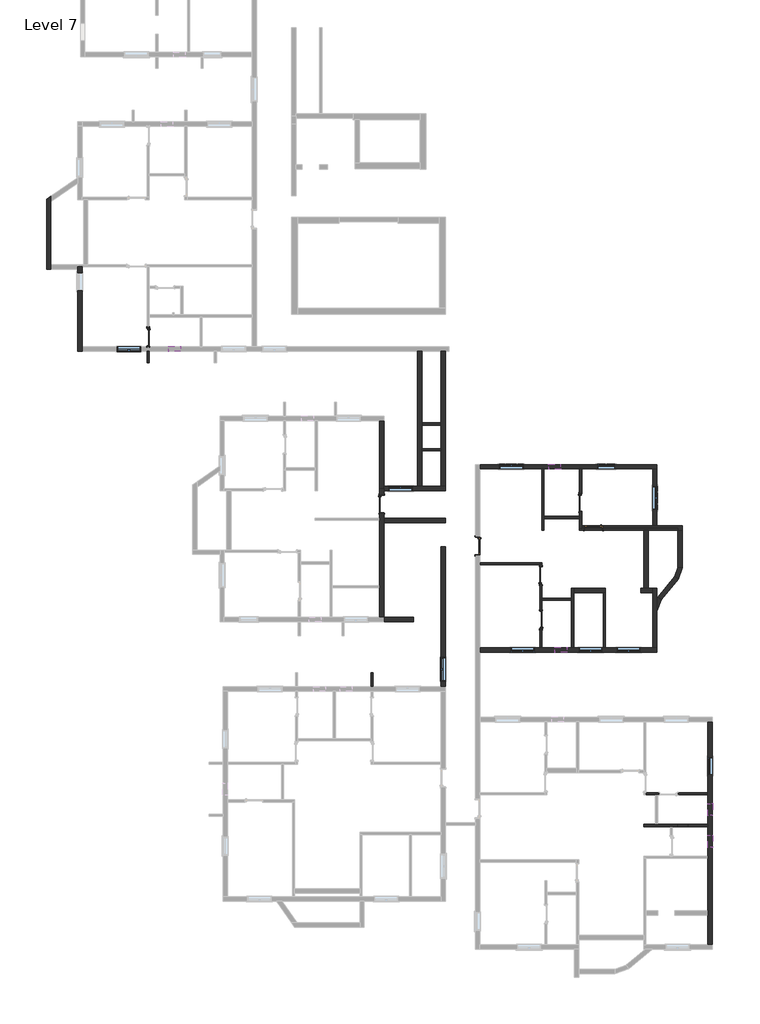
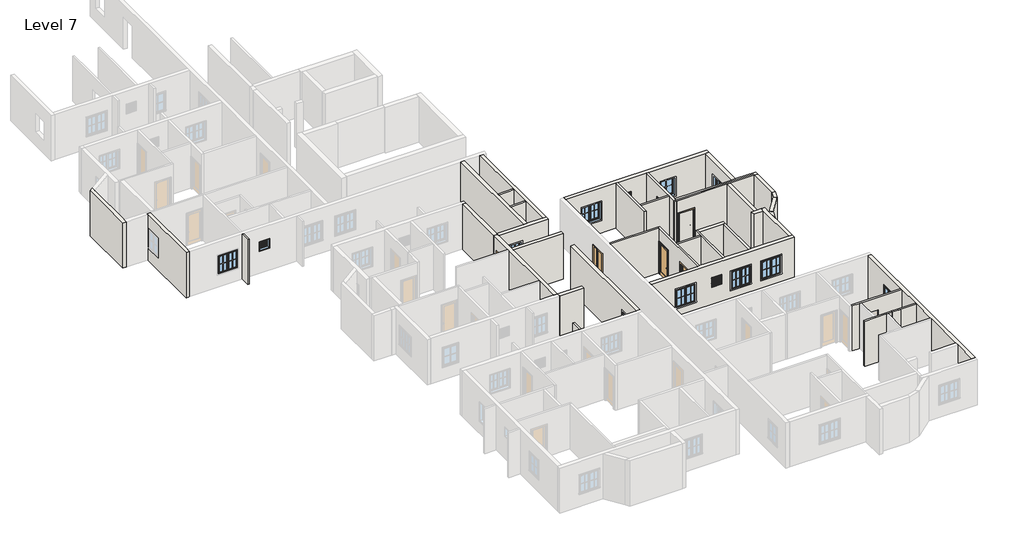
# One storey, part 3 of 7: 39 walls, 15 windows, 7 doors.
"""IFC4 building model written with IfcOpenShell, lengths in millimetres."""

from ifc_helpers import new_model, si_unit, point, frame, frame_2d, origin, place, context, project, spatial, polyline, circle_curve, trimmed, segment, composite_curve, outline, extrude, faceted_brep, transform, mapped, element, save
from components import door_3c6ab76a, door_a3feeac7, door_3b97b8e7, door_868ee8a9, window_272f20d6, window_casement_double_4_x_4_af3140d2, window_f2d8fef0

model = new_model("IFC4")

# Units and contexts
model_context = context("Model", 3, world=origin())
ifc_project = project(units=[si_unit("LENGTHUNIT", "METRE", prefix="MILLI")], contexts=[model_context])

# Site, building, storey
site = spatial("IfcSite", under=ifc_project)
building = spatial("IfcBuilding", under=site)
storey = spatial("IfcBuildingStorey", under=building, Name="Level 7", Elevation=9601.2)

# Doors
placement = place(None, origin())
door_shape = door_3c6ab76a(model_context)
element("IfcDoor", 1, ObjectType="Door-Interior-Single-1_Panel-Wood : 2'6\" x 7' door", at=placement, inside=storey, context=model_context, shape_type="MappedRepresentation", body=[
    mapped(door_shape, transform((-11252.4759469, 2064.0461172, 9601.2), x_axis=(0.0, -1.0, 0.0), y_axis=(1.0, 0.0, 0.0), z_axis=(0.0, 0.0, 1.0))),
])
door_2_shape = door_a3feeac7(model_context)
element("IfcDoor", 2, ObjectType="Door-Interior-Single-1_Panel-Wood : 2'6\" x 7' door", at=placement, inside=storey, context=model_context, shape_type="MappedRepresentation", body=[
    mapped(door_2_shape, transform((11042.3740531, -6465.2997229, 9601.2), x_axis=(0.0, -1.0, 0.0), y_axis=(1.0, 0.0, 0.0), z_axis=(0.0, 0.0, 1.0))),
])
element("IfcDoor", 3, ObjectType="Door-Interior-Single-1_Panel-Wood : 2'6\" x 7' door", at=placement, inside=storey, context=model_context, shape_type="MappedRepresentation", body=[
    mapped(door_2_shape, transform((9004.0240531, -12510.4997229, 9601.2), x_axis=(0.0, 1.0, 0.0), y_axis=(-1.0, 0.0, 0.0), z_axis=(0.0, 0.0, 1.0))),
])
element("IfcDoor", 4, ObjectType="Door-Interior-Single-1_Panel-Wood : 36\" x 84\"", at=placement, inside=storey, context=model_context, shape_type="MappedRepresentation", body=[
    mapped(door_shape, transform((8997.6740531, -10224.4997229, 9601.2), x_axis=(0.0, 1.0, 0.0), y_axis=(-1.0, 0.0, 0.0), z_axis=(0.0, 0.0, 1.0))),
])
door_3_shape = door_3b97b8e7(model_context)
element("IfcDoor", 5, ObjectType="Door-Interior-Single-1_Panel-Wood : 36\" x 84\"", at=placement, inside=storey, context=model_context, shape_type="MappedRepresentation", body=[
    mapped(door_3_shape, transform((5733.7740531, -8700.4997229, 9601.2), x_axis=(0.0, -1.0, 0.0), y_axis=(1.0, 0.0, 0.0), z_axis=(0.0, 0.0, 1.0))),
])
door_4_shape = door_868ee8a9(model_context)
element("IfcDoor", 6, ObjectType="Door-Interior-Single-1_Panel-Wood : 36\" x 84\"", at=placement, inside=storey, context=model_context, shape_type="MappedRepresentation", body=[
    mapped(door_4_shape, transform((787.1240531, -6537.0288828, 9601.2), x_axis=(0.0, -1.0, 0.0), y_axis=(1.0, 0.0, 0.0), z_axis=(0.0, 0.0, 1.0))),
])
element("IfcDoor", 7, ObjectType="Door-Interior-Single-1_Panel-Wood : 36\" x 84\"", at=placement, inside=storey, context=model_context, shape_type="MappedRepresentation", body=[
    mapped(door_4_shape, transform((11712.2990531, -7776.5747229, 9601.2), x_axis=(-1.0, 0.0, 0.0), y_axis=(0.0, -1.0, 0.0), z_axis=(0.0, 0.0, 1.0))),
])

# Walls
element("IfcWall", 8, ObjectType="4.5\" wall", at=placement, inside=storey, context=model_context, shape_type="SweptSolid", body=[
    extrude(outline(polyline([(-11312.8009469, 730.5461172), (-11312.8009469, 1340.1461172), (-11198.5009469, 1340.1461172), (-11198.5009469, 730.5461172), (-11312.8009469, 730.5461172)])), frame((0.0, 0.0, 9601.2), z_axis=(0.0, 0.0, 1.0), x_axis=(1.0, 0.0, 0.0)), (0.0, 0.0, 1.0), 3048.0),
])
element("IfcWall", 9, ObjectType="4.5\" wall", at=placement, inside=storey, context=model_context, shape_type="SweptSolid", body=[
    extrude(outline(polyline([(3850.9990531, -3803.3538828), (2860.3990531, -3803.3538828), (2860.3990531, -3689.0538828), (3850.9990531, -3689.0538828), (3850.9990531, -3803.3538828)])), frame((0.0, 0.0, 9601.2), z_axis=(0.0, 0.0, 1.0), x_axis=(1.0, 0.0, 0.0)), (0.0, 0.0, 1.0), 3048.0),
])
element("IfcWall", 10, ObjectType="4.5\" wall", at=placement, inside=storey, context=model_context, shape_type="SweptSolid", body=[
    extrude(outline(polyline([(2860.3990531, -2355.5538828), (3850.9990531, -2355.5538828), (3850.9990531, -2469.8538828), (2860.3990531, -2469.8538828), (2860.3990531, -2355.5538828)])), frame((0.0, 0.0, 9601.2), z_axis=(0.0, 0.0, 1.0), x_axis=(1.0, 0.0, 0.0)), (0.0, 0.0, 1.0), 3048.0),
])
element("IfcWall", 11, ObjectType="4.5\" wall", at=placement, inside=storey, context=model_context, shape_type="SweptSolid", body=[
    extrude(outline(polyline([(345.7990531, -15233.3538828), (345.7990531, -15957.2538828), (231.4990531, -15957.2538828), (231.4990531, -15233.3538828), (345.7990531, -15233.3538828)])), frame((0.0, 0.0, 9601.2), z_axis=(0.0, 0.0, 1.0), x_axis=(1.0, 0.0, 0.0)), (0.0, 0.0, 1.0), 3048.0),
])
element("IfcWall", 12, ObjectType="4.5\" wall", at=placement, inside=storey, context=model_context, shape_type="Brep", body=[
    faceted_brep([(17617.7990531, -21521.1497229, 12649.2), (15026.9990531, -21521.1497229, 12649.2), (14912.6990531, -21521.1497229, 12649.2), (14417.3990531, -21521.1497229, 12649.2), (14417.3990531, -21521.1497229, 9601.2), (14912.6990531, -21521.1497229, 9601.2), (15026.9990531, -21521.1497229, 9601.2), (15096.8490531, -21521.1497229, 9601.2), (15096.8490531, -21521.1497229, 11760.2), (16062.0490531, -21521.1497229, 11760.2), (16062.0490531, -21521.1497229, 9601.2), (17617.7990531, -21521.1497229, 9601.2), (14417.3990531, -21406.8497229, 12649.2), (17617.7990531, -21406.8497229, 12649.2), (17617.7990531, -21406.8497229, 9601.2), (16062.0490531, -21406.8497229, 9601.2), (16062.0490531, -21406.8497229, 11760.2), (15096.8490531, -21406.8497229, 11760.2), (15096.8490531, -21406.8497229, 9601.2), (14417.3990531, -21406.8497229, 9601.2)], [[[0, 1, 2, 3, 4, 5, 6, 7, 8, 9, 10, 11]], [[12, 13, 14, 15, 16, 17, 18, 19]], [[14, 11, 10, 15]], [[4, 19, 18, 7, 6, 5]], [[3, 2, 1, 0, 13, 12]], [[0, 11, 14, 13]], [[4, 3, 12, 19]], [[17, 8, 7, 18]], [[8, 17, 16, 9]], [[9, 16, 15, 10]]]),
])
element("IfcWall", 13, ObjectType="4.5\" wall", at=placement, inside=storey, context=model_context, shape_type="SweptSolid", body=[
    extrude(outline(polyline([(16055.6990531, -23045.1497229), (16589.0990531, -23045.1497229), (16589.0990531, -23159.4497229), (16055.6990531, -23159.4497229), (16055.6990531, -23045.1497229)])), frame((0.0, 0.0, 9601.2), z_axis=(0.0, 0.0, 1.0), x_axis=(1.0, 0.0, 0.0)), (0.0, 0.0, 1.0), 3048.0),
])
element("IfcWall", 14, ObjectType="4.5\" wall", at=placement, inside=storey, context=model_context, shape_type="Brep", body=[
    faceted_brep([(17617.7990531, -23045.1497229, 9601.2), (15026.9990531, -23045.1497229, 9601.2), (14912.6990531, -23045.1497229, 9601.2), (14303.0990531, -23045.1497229, 9601.2), (14303.0990531, -23045.1497229, 12649.2), (14912.6990531, -23045.1497229, 12649.2), (15026.9990531, -23045.1497229, 12649.2), (17617.7990531, -23045.1497229, 12649.2), (17617.7990531, -23159.4497229, 9601.2), (17617.7990531, -23159.4497229, 12649.2), (15788.9990531, -23159.4497229, 12649.2), (15674.6990531, -23159.4497229, 12649.2), (14303.0990531, -23159.4497229, 12649.2), (14303.0990531, -23159.4497229, 9601.2), (15674.6990531, -23159.4497229, 9601.2), (15788.9990531, -23159.4497229, 9601.2)], [[[0, 1, 2, 3, 4, 5, 6, 7]], [[8, 9, 10, 11, 12, 13, 14, 15]], [[3, 2, 1, 0, 8, 15, 14, 13]], [[4, 3, 13, 12]], [[7, 6, 5, 4, 12, 11, 10, 9]], [[0, 7, 9, 8]]]),
])
element("IfcWall", 15, ObjectType="4.5\" wall", at=placement, inside=storey, context=model_context, shape_type="Brep", body=[
    faceted_brep([(10988.3990531, -7894.0497229, 9601.2), (14303.0990531, -7894.0497229, 9601.2), (14531.6990531, -7894.0497229, 9601.2), (16055.6990531, -7894.0497229, 9601.2), (16055.6990531, -7894.0497229, 12649.2), (14531.6990531, -7894.0497229, 12649.2), (14303.0990531, -7894.0497229, 12649.2), (10988.3990531, -7894.0497229, 12649.2), (10988.3990531, -7779.7497229, 9601.2), (10988.3990531, -7779.7497229, 12649.2), (11102.6990531, -7779.7497229, 12649.2), (16055.6990531, -7779.7497229, 12649.2), (16055.6990531, -7779.7497229, 9601.2), (11102.6990531, -7779.7497229, 9601.2)], [[[0, 1, 2, 3, 4, 5, 6, 7]], [[8, 9, 10, 11, 12, 13]], [[3, 2, 1, 0, 8, 13, 12]], [[7, 6, 5, 4, 11, 10, 9]], [[0, 7, 9, 8]], [[4, 3, 12, 11]]]),
])
element("IfcWall", 16, ObjectType="4.5\" wall", at=placement, inside=storey, context=model_context, shape_type="Brep", body=[
    faceted_brep([(10696.2990531, -13939.2497229, 9601.2), (10696.2990531, -11119.8497229, 9601.2), (10696.2990531, -10891.2497229, 9601.2), (10696.2990531, -10891.2497229, 12649.2), (10696.2990531, -11119.8497229, 12649.2), (10696.2990531, -13939.2497229, 12649.2), (10581.9990531, -13939.2497229, 9601.2), (10581.9990531, -13939.2497229, 12649.2), (10581.9990531, -11500.8497229, 12649.2), (10581.9990531, -11386.5497229, 12649.2), (10581.9990531, -10891.2497229, 12649.2), (10581.9990531, -10891.2497229, 9601.2), (10581.9990531, -11386.5497229, 9601.2), (10581.9990531, -11500.8497229, 9601.2)], [[[0, 1, 2, 3, 4, 5]], [[6, 7, 8, 9, 10, 11, 12, 13]], [[2, 1, 0, 6, 13, 12, 11]], [[5, 4, 3, 10, 9, 8, 7]], [[0, 5, 7, 6]], [[3, 2, 11, 10]]]),
])
element("IfcWall", 17, ObjectType="4.5\" wall", at=placement, inside=storey, context=model_context, shape_type="SweptSolid", body=[
    extrude(outline(polyline([(9057.9990531, -11386.5497229), (10581.9990531, -11386.5497229), (10581.9990531, -11500.8497229), (9057.9990531, -11500.8497229), (9057.9990531, -11386.5497229)])), frame((0.0, 0.0, 9601.2), z_axis=(0.0, 0.0, 1.0), x_axis=(1.0, 0.0, 0.0)), (0.0, 0.0, 1.0), 3048.0),
])
element("IfcWall", 18, ObjectType="4.5\" wall", at=placement, inside=storey, context=model_context, shape_type="Brep", body=[
    faceted_brep([(8943.6990531, -13939.2497229, 12649.2), (8943.6990531, -9672.0497229, 12649.2), (8943.6990531, -9557.7497229, 12649.2), (8943.6990531, -9557.7497229, 9601.2), (8943.6990531, -9672.0497229, 9601.2), (8943.6990531, -9741.8997229, 9601.2), (8943.6990531, -9741.8997229, 11760.2), (8943.6990531, -10707.0997229, 11760.2), (8943.6990531, -10707.0997229, 9601.2), (8943.6990531, -12027.8997229, 9601.2), (8943.6990531, -12027.8997229, 11760.2), (8943.6990531, -12993.0997229, 11760.2), (8943.6990531, -12993.0997229, 9601.2), (8943.6990531, -13939.2497229, 9601.2), (9057.9990531, -9557.7497229, 12649.2), (9057.9990531, -11386.5497229, 12649.2), (9057.9990531, -11500.8497229, 12649.2), (9057.9990531, -13939.2497229, 12649.2), (9057.9990531, -13939.2497229, 9601.2), (9057.9990531, -12993.0997229, 9601.2), (9057.9990531, -12993.0997229, 11760.2), (9057.9990531, -12027.8997229, 11760.2), (9057.9990531, -12027.8997229, 9601.2), (9057.9990531, -11500.8497229, 9601.2), (9057.9990531, -11386.5497229, 9601.2), (9057.9990531, -10707.0997229, 9601.2), (9057.9990531, -10707.0997229, 11760.2), (9057.9990531, -9741.8997229, 11760.2), (9057.9990531, -9741.8997229, 9601.2), (9057.9990531, -9557.7497229, 9601.2)], [[[0, 1, 2, 3, 4, 5, 6, 7, 8, 9, 10, 11, 12, 13]], [[14, 15, 16, 17, 18, 19, 20, 21, 22, 23, 24, 25, 26, 27, 28, 29]], [[18, 13, 12, 19]], [[3, 29, 28, 5, 4]], [[22, 9, 8, 25, 24, 23]], [[2, 1, 0, 17, 16, 15, 14]], [[0, 13, 18, 17]], [[3, 2, 14, 29]], [[21, 10, 9, 22]], [[10, 21, 20, 11]], [[11, 20, 19, 12]], [[27, 6, 5, 28]], [[6, 27, 26, 7]], [[7, 26, 25, 8]]]),
])
element("IfcWall", 19, ObjectType="4.5\" wall", at=placement, inside=storey, context=model_context, shape_type="SweptSolid", body=[
    extrude(outline(polyline([(8943.6990531, -9672.0497229), (5844.8990531, -9672.0497229), (5844.8990531, -9557.7497229), (8943.6990531, -9557.7497229), (8943.6990531, -9672.0497229)])), frame((0.0, 0.0, 9601.2), z_axis=(0.0, 0.0, 1.0), x_axis=(1.0, 0.0, 0.0)), (0.0, 0.0, 1.0), 3048.0),
])
element("IfcWall", 20, ObjectType="4.5\" wall", at=placement, inside=storey, context=model_context, shape_type="Brep", body=[
    faceted_brep([(9045.2990531, -4731.7497229, 9601.2), (9045.2990531, -7894.0497229, 9601.2), (9045.2990531, -7894.0497229, 12649.2), (9045.2990531, -4731.7497229, 12649.2), (9159.5990531, -4731.7497229, 9601.2), (9159.5990531, -4731.7497229, 12649.2), (9159.5990531, -7170.1497229, 12649.2), (9159.5990531, -7284.4497229, 12649.2), (9159.5990531, -7894.0497229, 12649.2), (9159.5990531, -7894.0497229, 9601.2), (9159.5990531, -7284.4497229, 9601.2), (9159.5990531, -7170.1497229, 9601.2)], [[[0, 1, 2, 3]], [[4, 5, 6, 7, 8, 9, 10, 11]], [[1, 0, 4, 11, 10, 9]], [[2, 1, 9, 8]], [[3, 2, 8, 7, 6, 5]], [[0, 3, 5, 4]]]),
])
element("IfcWall", 21, ObjectType="4.5\" wall", at=placement, inside=storey, context=model_context, shape_type="Brep", body=[
    faceted_brep([(10988.3990531, -7779.7497229, 12649.2), (10988.3990531, -7284.4497229, 12649.2), (10988.3990531, -7170.1497229, 12649.2), (10988.3990531, -4731.7497229, 12649.2), (10988.3990531, -4731.7497229, 9601.2), (10988.3990531, -5982.6997229, 9601.2), (10988.3990531, -5982.6997229, 11760.2), (10988.3990531, -6947.8997229, 11760.2), (10988.3990531, -6947.8997229, 9601.2), (10988.3990531, -7170.1497229, 9601.2), (10988.3990531, -7284.4497229, 9601.2), (10988.3990531, -7779.7497229, 9601.2), (11102.6990531, -4731.7497229, 12649.2), (11102.6990531, -7665.4497229, 12649.2), (11102.6990531, -7779.7497229, 12649.2), (11102.6990531, -7779.7497229, 9601.2), (11102.6990531, -7665.4497229, 9601.2), (11102.6990531, -6947.8997229, 9601.2), (11102.6990531, -6947.8997229, 11760.2), (11102.6990531, -5982.6997229, 11760.2), (11102.6990531, -5982.6997229, 9601.2), (11102.6990531, -4731.7497229, 9601.2)], [[[0, 1, 2, 3, 4, 5, 6, 7, 8, 9, 10, 11]], [[12, 13, 14, 15, 16, 17, 18, 19, 20, 21]], [[4, 21, 20, 5]], [[15, 11, 10, 9, 8, 17, 16]], [[3, 2, 1, 0, 14, 13, 12]], [[4, 3, 12, 21]], [[0, 11, 15, 14]], [[7, 18, 17, 8]], [[18, 7, 6, 19]], [[19, 6, 5, 20]]]),
])
element("IfcWall", 22, ObjectType="4.5\" wall", at=placement, inside=storey, context=model_context, shape_type="SweptSolid", body=[
    extrude(outline(polyline([(10988.3990531, -7284.4497229), (9159.5990531, -7284.4497229), (9159.5990531, -7170.1497229), (10988.3990531, -7170.1497229), (10988.3990531, -7284.4497229)])), frame((0.0, 0.0, 9601.2), z_axis=(0.0, 0.0, 1.0), x_axis=(1.0, 0.0, 0.0)), (0.0, 0.0, 1.0), 3048.0),
])
element("IfcWall", 23, ObjectType="4.5\" wall", at=placement, inside=storey, context=model_context, shape_type="SweptSolid", body=[
    extrude(outline(polyline([(12220.2990531, -13939.2497229), (12220.2990531, -11119.8497229), (12334.5990531, -11119.8497229), (12334.5990531, -13939.2497229), (12220.2990531, -13939.2497229)])), frame((0.0, 0.0, 9601.2), z_axis=(0.0, 0.0, 1.0), x_axis=(1.0, 0.0, 0.0)), (0.0, 0.0, 1.0), 3048.0),
])
element("IfcWall", 24, ObjectType="9\"", at=placement, inside=storey, context=model_context, shape_type="Brep", body=[
    faceted_brep([(-14894.2009469, 5683.5461172, 9601.2), (-14894.2009469, 5569.2461172, 9601.2), (-14894.2009469, 1340.1461172, 9601.2), (-14894.2009469, 1340.1461172, 12649.2), (-14894.2009469, 5569.2461172, 12649.2), (-14894.2009469, 5683.5461172, 12649.2), (-14894.2009469, 5378.7461172, 11734.8), (-14894.2009469, 4464.3461172, 11734.8), (-14894.2009469, 4464.3461172, 10515.6), (-14894.2009469, 5378.7461172, 10515.6), (-14665.6009469, 5683.5461172, 9601.2), (-14665.6009469, 5683.5461172, 12649.2), (-14665.6009469, 1568.7461172, 12649.2), (-14665.6009469, 1340.1461172, 12649.2), (-14665.6009469, 1340.1461172, 9601.2), (-14665.6009469, 1568.7461172, 9601.2), (-14665.6009469, 5378.7461172, 11734.8), (-14665.6009469, 5378.7461172, 10515.6), (-14665.6009469, 4464.3461172, 10515.6), (-14665.6009469, 4464.3461172, 11734.8)], [[[0, 1, 2, 3, 4, 5], [6, 7, 8, 9]], [[10, 11, 12, 13, 14, 15], [16, 17, 18, 19]], [[2, 1, 0, 10, 15, 14]], [[5, 4, 3, 13, 12, 11]], [[3, 2, 14, 13]], [[0, 5, 11, 10]], [[17, 16, 6, 9]], [[18, 17, 9, 8]], [[19, 18, 8, 7]], [[16, 19, 7, 6]]]),
])
element("IfcWall", 25, ObjectType="9\"", at=placement, inside=storey, context=model_context, shape_type="Brep", body=[
    faceted_brep([(904.5990531, -5746.4538828, 9601.2), (904.5990531, -5632.1538828, 9601.2), (904.5990531, -2241.2538828, 9601.2), (904.5990531, -2241.2538828, 12649.2), (904.5990531, -5632.1538828, 12649.2), (904.5990531, -5746.4538828, 12649.2), (675.9990531, -5746.4538828, 9601.2), (675.9990531, -5746.4538828, 12649.2), (675.9990531, -2241.2538828, 12649.2), (675.9990531, -2241.2538828, 9601.2)], [[[0, 1, 2, 3, 4, 5]], [[6, 7, 8, 9]], [[2, 1, 0, 6, 9]], [[5, 4, 3, 8, 7]], [[0, 5, 7, 6]], [[3, 2, 9, 8]]]),
])
element("IfcWall", 26, ObjectType="9\"", at=placement, inside=storey, context=model_context, shape_type="Brep", body=[
    faceted_brep([(904.5990531, -5746.4538828, 9601.2), (904.5990531, -5746.4538828, 12649.2), (904.5990531, -5860.7538828, 12649.2), (904.5990531, -7270.4538828, 12649.2), (904.5990531, -7499.0538828, 12649.2), (904.5990531, -12375.8538828, 12649.2), (904.5990531, -12375.8538828, 9601.2), (904.5990531, -7499.0538828, 9601.2), (904.5990531, -7270.4538828, 9601.2), (904.5990531, -7019.6288828, 9601.2), (904.5990531, -7019.6288828, 11760.2), (904.5990531, -6054.4288828, 11760.2), (904.5990531, -6054.4288828, 9601.2), (904.5990531, -5860.7538828, 9601.2), (675.9990531, -5746.4538828, 12649.2), (675.9990531, -5746.4538828, 9601.2), (675.9990531, -6054.4288828, 9601.2), (675.9990531, -6054.4288828, 11760.2), (675.9990531, -7019.6288828, 11760.2), (675.9990531, -7019.6288828, 9601.2), (675.9990531, -7270.4538828, 9601.2), (675.9990531, -7384.7538828, 9601.2), (675.9990531, -10737.5538828, 9601.2), (675.9990531, -10851.8538828, 9601.2), (675.9990531, -12375.8538828, 9601.2), (675.9990531, -12375.8538828, 12649.2), (675.9990531, -10851.8538828, 12649.2), (675.9990531, -10737.5538828, 12649.2), (675.9990531, -7384.7538828, 12649.2), (675.9990531, -7270.4538828, 12649.2)], [[[0, 1, 2, 3, 4, 5, 6, 7, 8, 9, 10, 11, 12, 13]], [[14, 15, 16, 17, 18, 19, 20, 21, 22, 23, 24, 25, 26, 27, 28, 29]], [[6, 24, 23, 22, 21, 20, 19, 9, 8, 7]], [[15, 0, 13, 12, 16]], [[1, 0, 15, 14]], [[5, 4, 3, 2, 1, 14, 29, 28, 27, 26, 25]], [[6, 5, 25, 24]], [[18, 10, 9, 19]], [[10, 18, 17, 11]], [[11, 17, 16, 12]]]),
])
element("IfcWall", 27, ObjectType="9\"", at=placement, inside=storey, context=model_context, shape_type="SweptSolid", body=[
    extrude(outline(polyline([(904.5990531, -7270.4538828), (4079.5990531, -7270.4538828), (4079.5990531, -7499.0538828), (904.5990531, -7499.0538828), (904.5990531, -7270.4538828)])), frame((0.0, 0.0, 9601.2), z_axis=(0.0, 0.0, 1.0), x_axis=(1.0, 0.0, 0.0)), (0.0, 0.0, 1.0), 3048.0),
])
element("IfcWall", 28, ObjectType="9\"", at=placement, inside=storey, context=model_context, shape_type="Brep", body=[
    faceted_brep([(904.5990531, -5860.7538828, 9601.2), (4079.5990531, -5860.7538828, 9601.2), (4079.5990531, -5860.7538828, 12649.2), (904.5990531, -5860.7538828, 12649.2), (2377.7990531, -5860.7538828, 11734.8), (2377.7990531, -5860.7538828, 10515.6), (1158.5990531, -5860.7538828, 10515.6), (1158.5990531, -5860.7538828, 11734.8), (904.5990531, -5632.1538828, 9601.2), (904.5990531, -5632.1538828, 12649.2), (2631.7990531, -5632.1538828, 12649.2), (2860.3990531, -5632.1538828, 12649.2), (3850.9990531, -5632.1538828, 12649.2), (4079.5990531, -5632.1538828, 12649.2), (4079.5990531, -5632.1538828, 9601.2), (3850.9990531, -5632.1538828, 9601.2), (2860.3990531, -5632.1538828, 9601.2), (2631.7990531, -5632.1538828, 9601.2), (2377.7990531, -5632.1538828, 11734.8), (1158.5990531, -5632.1538828, 11734.8), (1158.5990531, -5632.1538828, 10515.6), (2377.7990531, -5632.1538828, 10515.6), (904.5990531, -5746.4538828, 9601.2), (904.5990531, -5746.4538828, 12649.2)], [[[0, 1, 2, 3], [4, 5, 6, 7]], [[8, 9, 10, 11, 12, 13, 14, 15, 16, 17], [18, 19, 20, 21]], [[1, 0, 22, 8, 17, 16, 15, 14]], [[3, 2, 13, 12, 11, 10, 9, 23]], [[0, 3, 23, 9, 8, 22]], [[2, 1, 14, 13]], [[5, 4, 18, 21]], [[6, 5, 21, 20]], [[7, 6, 20, 19]], [[4, 7, 19, 18]]]),
])
element("IfcWall", 29, ObjectType="9\"", at=placement, inside=storey, context=model_context, shape_type="Brep", body=[
    faceted_brep([(2631.7990531, 1340.1461172, 9601.2), (2631.7990531, -5632.1538828, 9601.2), (2631.7990531, -5632.1538828, 12649.2), (2631.7990531, 1340.1461172, 12649.2), (2860.3990531, 1340.1461172, 9601.2), (2860.3990531, 1340.1461172, 12649.2), (2860.3990531, -2355.5538828, 12649.2), (2860.3990531, -2469.8538828, 12649.2), (2860.3990531, -3689.0538828, 12649.2), (2860.3990531, -3803.3538828, 12649.2), (2860.3990531, -5632.1538828, 12649.2), (2860.3990531, -5632.1538828, 9601.2), (2860.3990531, -3803.3538828, 9601.2), (2860.3990531, -3689.0538828, 9601.2), (2860.3990531, -2469.8538828, 9601.2), (2860.3990531, -2355.5538828, 9601.2)], [[[0, 1, 2, 3]], [[4, 5, 6, 7, 8, 9, 10, 11, 12, 13, 14, 15]], [[1, 0, 4, 15, 14, 13, 12, 11]], [[3, 2, 10, 9, 8, 7, 6, 5]], [[0, 3, 5, 4]], [[2, 1, 11, 10]]]),
])
element("IfcWall", 30, ObjectType="9\"", at=placement, inside=storey, context=model_context, shape_type="Brep", body=[
    faceted_brep([(4079.5990531, -5632.1538828, 9601.2), (4079.5990531, 1340.1461172, 9601.2), (4079.5990531, 1340.1461172, 12649.2), (4079.5990531, -5632.1538828, 12649.2), (3850.9990531, -5632.1538828, 9601.2), (3850.9990531, -5632.1538828, 12649.2), (3850.9990531, -3803.3538828, 12649.2), (3850.9990531, -3689.0538828, 12649.2), (3850.9990531, -2469.8538828, 12649.2), (3850.9990531, -2355.5538828, 12649.2), (3850.9990531, 1340.1461172, 12649.2), (3850.9990531, 1340.1461172, 9601.2), (3850.9990531, -2355.5538828, 9601.2), (3850.9990531, -2469.8538828, 9601.2), (3850.9990531, -3689.0538828, 9601.2), (3850.9990531, -3803.3538828, 9601.2)], [[[0, 1, 2, 3]], [[4, 5, 6, 7, 8, 9, 10, 11, 12, 13, 14, 15]], [[1, 0, 4, 15, 14, 13, 12, 11]], [[3, 2, 10, 9, 8, 7, 6, 5]], [[2, 1, 11, 10]], [[0, 3, 5, 4]]]),
])
element("IfcWall", 31, ObjectType="9\"", at=placement, inside=storey, context=model_context, shape_type="SweptSolid", body=[
    extrude(outline(polyline([(904.5990531, -12375.8538828), (2441.2990531, -12375.8538828), (2441.2990531, -12604.4538828), (904.5990531, -12604.4538828), (904.5990531, -12375.8538828)])), frame((0.0, 0.0, 9601.2), z_axis=(0.0, 0.0, 1.0), x_axis=(1.0, 0.0, 0.0)), (0.0, 0.0, 1.0), 3048.0),
])
element("IfcWall", 32, ObjectType="9\"", at=placement, inside=storey, context=model_context, shape_type="Brep", body=[
    faceted_brep([(17617.7990531, -17749.2497229, 9601.2), (17617.7990531, -21406.8497229, 9601.2), (17617.7990531, -21521.1497229, 9601.2), (17617.7990531, -23045.1497229, 9601.2), (17617.7990531, -23159.4497229, 9601.2), (17617.7990531, -24683.4497229, 9601.2), (17617.7990531, -24797.7497229, 9601.2), (17617.7990531, -27502.8497229, 9601.2), (17617.7990531, -27731.4497229, 9601.2), (17617.7990531, -29255.4497229, 9601.2), (17617.7990531, -29255.4497229, 12649.2), (17617.7990531, -27731.4497229, 12649.2), (17617.7990531, -27502.8497229, 12649.2), (17617.7990531, -24797.7497229, 12649.2), (17617.7990531, -24683.4497229, 12649.2), (17617.7990531, -23159.4497229, 12649.2), (17617.7990531, -23045.1497229, 12649.2), (17617.7990531, -21521.1497229, 12649.2), (17617.7990531, -21406.8497229, 12649.2), (17617.7990531, -17749.2497229, 12649.2), (17617.7990531, -22587.9497229, 11734.8), (17617.7990531, -22587.9497229, 11125.2), (17617.7990531, -21978.3497229, 11125.2), (17617.7990531, -21978.3497229, 11734.8), (17617.7990531, -23616.6497229, 11734.8), (17617.7990531, -24226.2497229, 11734.8), (17617.7990531, -24226.2497229, 11125.2), (17617.7990531, -23616.6497229, 11125.2), (17617.7990531, -19584.3997229, 11734.8), (17617.7990531, -20498.7997229, 11734.8), (17617.7990531, -20498.7997229, 10515.6), (17617.7990531, -19584.3997229, 10515.6), (17846.3990531, -17749.2497229, 9601.2), (17846.3990531, -17749.2497229, 12649.2), (17846.3990531, -29255.4497229, 12649.2), (17846.3990531, -29255.4497229, 9601.2), (17846.3990531, -22587.9497229, 11734.8), (17846.3990531, -21978.3497229, 11734.8), (17846.3990531, -21978.3497229, 11125.2), (17846.3990531, -22587.9497229, 11125.2), (17846.3990531, -23616.6497229, 11734.8), (17846.3990531, -23616.6497229, 11125.2), (17846.3990531, -24226.2497229, 11125.2), (17846.3990531, -24226.2497229, 11734.8), (17846.3990531, -19584.3997229, 11734.8), (17846.3990531, -19584.3997229, 10515.6), (17846.3990531, -20498.7997229, 10515.6), (17846.3990531, -20498.7997229, 11734.8)], [[[0, 1, 2, 3, 4, 5, 6, 7, 8, 9, 10, 11, 12, 13, 14, 15, 16, 17, 18, 19], [20, 21, 22, 23], [24, 25, 26, 27], [28, 29, 30, 31]], [[32, 33, 34, 35], [36, 37, 38, 39], [40, 41, 42, 43], [44, 45, 46, 47]], [[9, 8, 7, 6, 5, 4, 3, 2, 1, 0, 32, 35]], [[19, 18, 17, 16, 15, 14, 13, 12, 11, 10, 34, 33]], [[0, 19, 33, 32]], [[10, 9, 35, 34]], [[21, 20, 36, 39]], [[22, 21, 39, 38]], [[23, 22, 38, 37]], [[20, 23, 37, 36]], [[41, 40, 24, 27]], [[42, 41, 27, 26]], [[43, 42, 26, 25]], [[40, 43, 25, 24]], [[45, 44, 28, 31]], [[46, 45, 31, 30]], [[47, 46, 30, 29]], [[44, 47, 29, 28]]]),
])
element("IfcWall", 33, ObjectType="9\"", at=placement, inside=storey, context=model_context, shape_type="Brep", body=[
    faceted_brep([(5844.8990531, -14167.8497229, 9601.2), (14988.8990531, -14167.8497229, 9601.2), (14988.8990531, -14167.8497229, 12649.2), (5844.8990531, -14167.8497229, 12649.2), (10334.3490531, -14167.8497229, 11734.8), (10334.3490531, -14167.8497229, 11125.2), (9724.7490531, -14167.8497229, 11125.2), (9724.7490531, -14167.8497229, 11734.8), (12912.4490531, -14167.8497229, 11734.8), (14131.6490531, -14167.8497229, 11734.8), (14131.6490531, -14167.8497229, 10515.6), (12912.4490531, -14167.8497229, 10515.6), (10956.6490531, -14167.8497229, 11734.8), (12175.8490531, -14167.8497229, 11734.8), (12175.8490531, -14167.8497229, 10515.6), (10956.6490531, -14167.8497229, 10515.6), (7451.4490531, -14167.8497229, 11734.8), (8670.6490531, -14167.8497229, 11734.8), (8670.6490531, -14167.8497229, 10515.6), (7451.4490531, -14167.8497229, 10515.6), (5844.8990531, -13939.2497229, 9601.2), (5844.8990531, -13939.2497229, 12649.2), (8943.6990531, -13939.2497229, 12649.2), (9057.9990531, -13939.2497229, 12649.2), (10581.9990531, -13939.2497229, 12649.2), (10696.2990531, -13939.2497229, 12649.2), (12220.2990531, -13939.2497229, 12649.2), (12334.5990531, -13939.2497229, 12649.2), (14760.2990531, -13939.2497229, 12649.2), (14988.8990531, -13939.2497229, 12649.2), (14988.8990531, -13939.2497229, 9601.2), (14760.2990531, -13939.2497229, 9601.2), (12334.5990531, -13939.2497229, 9601.2), (12220.2990531, -13939.2497229, 9601.2), (10696.2990531, -13939.2497229, 9601.2), (10581.9990531, -13939.2497229, 9601.2), (9057.9990531, -13939.2497229, 9601.2), (8943.6990531, -13939.2497229, 9601.2), (10334.3490531, -13939.2497229, 11734.8), (9724.7490531, -13939.2497229, 11734.8), (9724.7490531, -13939.2497229, 11125.2), (10334.3490531, -13939.2497229, 11125.2), (12912.4490531, -13939.2497229, 11734.8), (12912.4490531, -13939.2497229, 10515.6), (14131.6490531, -13939.2497229, 10515.6), (14131.6490531, -13939.2497229, 11734.8), (10956.6490531, -13939.2497229, 11734.8), (10956.6490531, -13939.2497229, 10515.6), (12175.8490531, -13939.2497229, 10515.6), (12175.8490531, -13939.2497229, 11734.8), (7451.4490531, -13939.2497229, 11734.8), (7451.4490531, -13939.2497229, 10515.6), (8670.6490531, -13939.2497229, 10515.6), (8670.6490531, -13939.2497229, 11734.8)], [[[0, 1, 2, 3], [4, 5, 6, 7], [8, 9, 10, 11], [12, 13, 14, 15], [16, 17, 18, 19]], [[20, 21, 22, 23, 24, 25, 26, 27, 28, 29, 30, 31, 32, 33, 34, 35, 36, 37], [38, 39, 40, 41], [42, 43, 44, 45], [46, 47, 48, 49], [50, 51, 52, 53]], [[1, 0, 20, 37, 36, 35, 34, 33, 32, 31, 30]], [[3, 2, 29, 28, 27, 26, 25, 24, 23, 22, 21]], [[0, 3, 21, 20]], [[2, 1, 30, 29]], [[5, 4, 38, 41]], [[6, 5, 41, 40]], [[7, 6, 40, 39]], [[4, 7, 39, 38]], [[43, 42, 8, 11]], [[44, 43, 11, 10]], [[45, 44, 10, 9]], [[42, 45, 9, 8]], [[47, 46, 12, 15]], [[48, 47, 15, 14]], [[49, 48, 14, 13]], [[46, 49, 13, 12]], [[51, 50, 16, 19]], [[52, 51, 19, 18]], [[53, 52, 18, 17]], [[50, 53, 17, 16]]]),
])
element("IfcWall", 34, ObjectType="9\"", at=placement, inside=storey, context=model_context, shape_type="SweptSolid", body=[
    extrude(outline(polyline([(-15957.2538828, 9601.2), (-15957.2538828, 12649.2), (-8732.9659091, 12649.2), (-8732.9659091, 9601.2), (-15957.2538828, 9601.2)]), holes=[polyline([(-14445.9538828, 11734.8), (-15665.1538828, 11734.8), (-15665.1538828, 10515.6), (-14445.9538828, 10515.6), (-14445.9538828, 11734.8)])]), frame((3850.9990531, 0.0, 0.0), z_axis=(1.0, 0.0, 0.0), x_axis=(0.0, 1.0, 0.0)), (0.0, 0.0, 1.0), 228.6),
])
element("IfcWall", 35, ObjectType="9\"", at=placement, inside=storey, context=model_context, shape_type="Brep", body=[
    faceted_brep([(5844.8990531, -4731.7497229, 9601.2), (9045.2990531, -4731.7497229, 9601.2), (9159.5990531, -4731.7497229, 9601.2), (10988.3990531, -4731.7497229, 9601.2), (11102.6990531, -4731.7497229, 9601.2), (14760.2990531, -4731.7497229, 9601.2), (14988.8990531, -4731.7497229, 9601.2), (14988.8990531, -4731.7497229, 12649.2), (14760.2990531, -4731.7497229, 12649.2), (11102.6990531, -4731.7497229, 12649.2), (10988.3990531, -4731.7497229, 12649.2), (9159.5990531, -4731.7497229, 12649.2), (9045.2990531, -4731.7497229, 12649.2), (5844.8990531, -4731.7497229, 12649.2), (10016.8490531, -4731.7497229, 11734.8), (10016.8490531, -4731.7497229, 11125.2), (9407.2490531, -4731.7497229, 11125.2), (9407.2490531, -4731.7497229, 11734.8), (12823.5490531, -4731.7497229, 11734.8), (12823.5490531, -4731.7497229, 10515.6), (11909.1490531, -4731.7497229, 10515.6), (11909.1490531, -4731.7497229, 11734.8), (8086.4490531, -4731.7497229, 11734.8), (8086.4490531, -4731.7497229, 10515.6), (6867.2490531, -4731.7497229, 10515.6), (6867.2490531, -4731.7497229, 11734.8), (5844.8990531, -4503.1497229, 9601.2), (5844.8990531, -4503.1497229, 12649.2), (14988.8990531, -4503.1497229, 12649.2), (14988.8990531, -4503.1497229, 9601.2), (10016.8490531, -4503.1497229, 11734.8), (9407.2490531, -4503.1497229, 11734.8), (9407.2490531, -4503.1497229, 11125.2), (10016.8490531, -4503.1497229, 11125.2), (12823.5490531, -4503.1497229, 11734.8), (11909.1490531, -4503.1497229, 11734.8), (11909.1490531, -4503.1497229, 10515.6), (12823.5490531, -4503.1497229, 10515.6), (8086.4490531, -4503.1497229, 11734.8), (6867.2490531, -4503.1497229, 11734.8), (6867.2490531, -4503.1497229, 10515.6), (8086.4490531, -4503.1497229, 10515.6)], [[[0, 1, 2, 3, 4, 5, 6, 7, 8, 9, 10, 11, 12, 13], [14, 15, 16, 17], [18, 19, 20, 21], [22, 23, 24, 25]], [[26, 27, 28, 29], [30, 31, 32, 33], [34, 35, 36, 37], [38, 39, 40, 41]], [[6, 5, 4, 3, 2, 1, 0, 26, 29]], [[13, 12, 11, 10, 9, 8, 7, 28, 27]], [[7, 6, 29, 28]], [[0, 13, 27, 26]], [[15, 14, 30, 33]], [[16, 15, 33, 32]], [[17, 16, 32, 31]], [[14, 17, 31, 30]], [[19, 18, 34, 37]], [[20, 19, 37, 36]], [[21, 20, 36, 35]], [[18, 21, 35, 34]], [[23, 22, 38, 41]], [[24, 23, 41, 40]], [[25, 24, 40, 39]], [[22, 25, 39, 38]]]),
])
element("IfcWall", 36, ObjectType="9\"", at=placement, inside=storey, context=model_context, shape_type="SweptSolid", body=[
    extrude(outline(polyline([(-7665.4497229, 9601.2), (-7665.4497229, 12649.2), (-4731.7497229, 12649.2), (-4731.7497229, 9601.2), (-7665.4497229, 9601.2)]), holes=[polyline([(-6836.7747229, 11734.8), (-6836.7747229, 10515.6), (-5617.5747229, 10515.6), (-5617.5747229, 11734.8), (-6836.7747229, 11734.8)])]), frame((14760.2990531, 0.0, 0.0), z_axis=(1.0, 0.0, 0.0), x_axis=(0.0, 1.0, 0.0)), (0.0, 0.0, 1.0), 228.6),
])
element("IfcWall", 37, ObjectType="9\"", at=placement, inside=storey, context=model_context, shape_type="Brep", body=[
    faceted_brep([(14988.8990531, -13939.2497229, 9601.2), (14988.8990531, -12059.0648255, 9601.2), (14988.8990531, -11373.2648255, 9601.2), (14988.8990531, -10891.2497229, 9601.2), (14988.8990531, -10891.2497229, 12649.2), (14988.8990531, -11373.2648255, 12649.2), (14988.8990531, -12059.0648255, 12649.2), (14988.8990531, -13939.2497229, 12649.2), (14760.2990531, -13939.2497229, 9601.2), (14760.2990531, -13939.2497229, 12649.2), (14760.2990531, -11119.8497229, 12649.2), (14760.2990531, -10891.2497229, 12649.2), (14760.2990531, -10891.2497229, 9601.2), (14760.2990531, -11119.8497229, 9601.2)], [[[0, 1, 2, 3, 4, 5, 6, 7]], [[8, 9, 10, 11, 12, 13]], [[3, 2, 1, 0, 8, 13, 12]], [[7, 6, 5, 4, 11, 10, 9]], [[0, 7, 9, 8]], [[4, 3, 12, 11]]]),
])
element("IfcWall", 38, ObjectType="9\"", at=placement, inside=storey, context=model_context, shape_type="SweptSolid", body=[
    extrude(outline(polyline([(14531.6990531, -7894.0497229), (14531.6990531, -10891.2497229), (14303.0990531, -10891.2497229), (14303.0990531, -7894.0497229), (14531.6990531, -7894.0497229)])), frame((0.0, 0.0, 9601.2), z_axis=(0.0, 0.0, 1.0), x_axis=(1.0, 0.0, 0.0)), (0.0, 0.0, 1.0), 3048.0),
])
element("IfcWall", 39, ObjectType="9\"", at=placement, inside=storey, context=model_context, shape_type="Brep", body=[
    faceted_brep([(10696.2990531, -11119.8497229, 9601.2), (12220.2990531, -11119.8497229, 9601.2), (12334.5990531, -11119.8497229, 9601.2), (12334.5990531, -11119.8497229, 12649.2), (12220.2990531, -11119.8497229, 12649.2), (10696.2990531, -11119.8497229, 12649.2), (10696.2990531, -10891.2497229, 9601.2), (10696.2990531, -10891.2497229, 12649.2), (12334.5990531, -10891.2497229, 12649.2), (12334.5990531, -10891.2497229, 9601.2)], [[[0, 1, 2, 3, 4, 5]], [[6, 7, 8, 9]], [[2, 1, 0, 6, 9]], [[5, 4, 3, 8, 7]], [[0, 5, 7, 6]], [[3, 2, 9, 8]]]),
])
element("IfcWall", 40, ObjectType="9\"", at=placement, inside=storey, context=model_context, shape_type="Brep", body=[
    faceted_brep([(14150.6990531, -11119.8497229, 9601.2), (14760.2990531, -11119.8497229, 9601.2), (14760.2990531, -11119.8497229, 12649.2), (14150.6990531, -11119.8497229, 12649.2), (14150.6990531, -10891.2497229, 9601.2), (14150.6990531, -10891.2497229, 12649.2), (14303.0990531, -10891.2497229, 12649.2), (14531.6990531, -10891.2497229, 12649.2), (14760.2990531, -10891.2497229, 12649.2), (14760.2990531, -10891.2497229, 9601.2), (14531.6990531, -10891.2497229, 9601.2), (14303.0990531, -10891.2497229, 9601.2)], [[[0, 1, 2, 3]], [[4, 5, 6, 7, 8, 9, 10, 11]], [[1, 0, 4, 11, 10, 9]], [[3, 2, 8, 7, 6, 5]], [[0, 3, 5, 4]], [[2, 1, 9, 8]]]),
])
element("IfcWall", 41, ObjectType="9\"", at=placement, inside=storey, context=model_context, shape_type="Brep", body=[
    faceted_brep([(-16265.8009469, 5569.2461172, 9601.2), (-16265.8009469, 5797.8461172, 9601.2), (-16265.8009469, 9043.9661172, 9601.2), (-16265.8009469, 9323.0079786, 9601.2), (-16265.8009469, 9323.0079786, 12649.2), (-16265.8009469, 9043.9661172, 12649.2), (-16265.8009469, 5797.8461172, 12649.2), (-16265.8009469, 5569.2461172, 12649.2), (-16494.4009469, 5569.2461172, 9601.2), (-16494.4009469, 5569.2461172, 12649.2), (-16494.4009469, 9162.9879786, 12649.2), (-16494.4009469, 9162.9879786, 9601.2)], [[[0, 1, 2, 3, 4, 5, 6, 7]], [[8, 9, 10, 11]], [[3, 2, 1, 0, 8, 11]], [[7, 6, 5, 4, 10, 9]], [[4, 3, 11, 10]], [[0, 7, 9, 8]]]),
])
element("IfcWall", 42, ObjectType="9\"", at=placement, inside=storey, context=model_context, shape_type="Brep", body=[
    faceted_brep([(16284.2990531, -7894.0497229, 12649.2), (16055.6990531, -7894.0497229, 12649.2), (14531.6990531, -7894.0497229, 12649.2), (14303.0990531, -7894.0497229, 12649.2), (11102.6990531, -7894.0497229, 12649.2), (11102.6990531, -7894.0497229, 9601.2), (11229.6990531, -7894.0497229, 9601.2), (11229.6990531, -7894.0497229, 11760.2), (12194.8990531, -7894.0497229, 11760.2), (12194.8990531, -7894.0497229, 9601.2), (14303.0990531, -7894.0497229, 9601.2), (14531.6990531, -7894.0497229, 9601.2), (16055.6990531, -7894.0497229, 9601.2), (16284.2990531, -7894.0497229, 9601.2), (11102.6990531, -7665.4497229, 12649.2), (14760.2990531, -7665.4497229, 12649.2), (14988.8990531, -7665.4497229, 12649.2), (16284.2990531, -7665.4497229, 12649.2), (16284.2990531, -7665.4497229, 9601.2), (14988.8990531, -7665.4497229, 9601.2), (14760.2990531, -7665.4497229, 9601.2), (12194.8990531, -7665.4497229, 9601.2), (12194.8990531, -7665.4497229, 11760.2), (11229.6990531, -7665.4497229, 11760.2), (11229.6990531, -7665.4497229, 9601.2), (11102.6990531, -7665.4497229, 9601.2), (11102.6990531, -7779.7497229, 9601.2), (11102.6990531, -7779.7497229, 12649.2)], [[[0, 1, 2, 3, 4, 5, 6, 7, 8, 9, 10, 11, 12, 13]], [[14, 15, 16, 17, 18, 19, 20, 21, 22, 23, 24, 25]], [[5, 26, 25, 24, 6]], [[18, 13, 12, 11, 10, 9, 21, 20, 19]], [[4, 3, 2, 1, 0, 17, 16, 15, 14, 27]], [[5, 4, 27, 14, 25, 26]], [[0, 13, 18, 17]], [[23, 7, 6, 24]], [[7, 23, 22, 8]], [[8, 22, 21, 9]]]),
])
element("IfcWall", 43, ObjectType="9\"", at=placement, inside=storey, context=model_context, shape_type="SweptSolid", body=[
    extrude(outline(polyline([(16055.6990531, -9831.602777), (16055.6990531, -7894.0497229), (16284.2990531, -7894.0497229), (16284.2990531, -9831.602777), (16055.6990531, -9831.602777)])), frame((0.0, 0.0, 9601.2), z_axis=(0.0, 0.0, 1.0), x_axis=(1.0, 0.0, 0.0)), (0.0, 0.0, 1.0), 3048.0),
])
element("IfcWall", 44, ObjectType="9\"", at=placement, inside=storey, context=model_context, shape_type="SweptSolid", body=[
    extrude(outline(polyline([(16075.314258, -10413.4246987), (15197.8838481, -11477.2429037), (15021.5300469, -11331.7874233), (15898.9604568, -10267.9692183), (16075.314258, -10413.4246987)])), frame((0.0, 0.0, 9601.2), z_axis=(0.0, 0.0, 1.0), x_axis=(1.0, 0.0, 0.0)), (0.0, 0.0, 1.0), 3048.0),
])
element("IfcWall", 45, ObjectType="9\"", at=placement, inside=storey, context=model_context, shape_type="SweptSolid", body=[
    extrude(outline(composite_curve([segment(polyline([(16055.6990531, -9831.602777), (16284.2990531, -9831.602777)]), True, "CONTINUOUS"), segment(trimmed(circle_curve(frame_2d((15369.8990531, -9831.602777)), 914.4), [point((16284.2990531, -9831.602777))], [point((16075.314258, -10413.4246987))], False, "CARTESIAN"), True, "CONTINUOUS"), segment(polyline([(16075.314258, -10413.4246987), (15898.9604568, -10267.9692183)]), True, "CONTINUOUS"), segment(trimmed(circle_curve(frame_2d((15369.8990531, -9831.602777)), 685.8), [point((15898.9604568, -10267.9692183))], [point((16055.6990531, -9831.602777))], True, "CARTESIAN"), True, "CONTINUOUS")], self_intersect=False)), frame((0.0, 0.0, 9601.2), z_axis=(0.0, 0.0, 1.0), x_axis=(1.0, 0.0, 0.0)), (0.0, 0.0, 1.0), 3048.0),
])
element("IfcWall", 46, ObjectType="9\"", at=placement, inside=storey, context=model_context, shape_type="SweptSolid", body=[
    extrude(outline(composite_curve([segment(trimmed(circle_curve(frame_2d((-12059.0648255, 15903.2990531)), 1143.0), [point((-11331.7874233, 15021.5300469))], [point((-11373.2648255, 14988.8990531))], False, "CARTESIAN"), True, "CONTINUOUS"), segment(polyline([(-11373.2648255, 14988.8990531), (-12059.0648255, 14988.8990531)]), True, "CONTINUOUS"), segment(trimmed(circle_curve(frame_2d((-12059.0648255, 15903.2990531)), 914.4), [point((-12059.0648255, 14988.8990531))], [point((-11477.2429037, 15197.8838481))], True, "CARTESIAN"), True, "CONTINUOUS"), segment(polyline([(-11477.2429037, 15197.8838481), (-11331.7874233, 15021.5300469)]), True, "CONTINUOUS")], self_intersect=False)), frame((0.0, 0.0, 12649.2), z_axis=(0.0, 0.0, -1.0), x_axis=(0.0, 1.0, 0.0)), (0.0, 0.0, 1.0), 3048.0),
])

# Windows
window_shape = window_272f20d6(model_context)
element("IfcWindow", 47, ObjectType="Window-Awning-Single : 36\" x 48\"", at=placement, inside=storey, context=model_context, shape_type="MappedRepresentation", body=[
    mapped(window_shape, transform((12366.3490531, -4617.4497229, 9601.2), x_axis=(1.0, 0.0, 0.0), y_axis=(0.0, 1.0, 0.0), z_axis=(0.0, 0.0, 1.0))),
])
element("IfcWindow", 48, ObjectType="Window-Awning-Single : 36\" x 48\"", at=placement, inside=storey, context=model_context, shape_type="MappedRepresentation", body=[
    mapped(window_shape, transform((17732.0990531, -20041.5997229, 9601.2), x_axis=(0.0, 1.0, 0.0), y_axis=(-1.0, 0.0, 0.0), z_axis=(0.0, 0.0, 1.0))),
])
window_casement_double_4_x_4_shape = window_casement_double_4_x_4_af3140d2(model_context)
element("IfcWindow", 49, ObjectType="Window-Casement-Double : 4' x 4'", at=placement, inside=storey, context=model_context, shape_type="MappedRepresentation", body=[
    mapped(window_casement_double_4_x_4_shape, transform((14874.5990531, -6227.1747229, 9601.2), x_axis=(0.0, -1.0, 0.0), y_axis=(1.0, 0.0, 0.0), z_axis=(0.0, 0.0, 1.0))),
])
element("IfcWindow", 50, ObjectType="Window-Casement-Double : 4' x 4'", at=placement, inside=storey, context=model_context, shape_type="MappedRepresentation", body=[
    mapped(window_casement_double_4_x_4_shape, transform((7476.8490531, -4617.4497229, 9601.2), x_axis=(1.0, 0.0, 0.0), y_axis=(0.0, 1.0, 0.0), z_axis=(0.0, 0.0, 1.0))),
])
element("IfcWindow", 51, ObjectType="Window-Casement-Double : 4' x 4'", at=placement, inside=storey, context=model_context, shape_type="MappedRepresentation", body=[
    mapped(window_casement_double_4_x_4_shape, transform((13522.0490531, -14053.5497229, 9601.2), x_axis=(-1.0, 0.0, 0.0), y_axis=(0.0, -1.0, 0.0), z_axis=(0.0, 0.0, 1.0))),
])
element("IfcWindow", 52, ObjectType="Window-Casement-Double : 4' x 4'", at=placement, inside=storey, context=model_context, shape_type="MappedRepresentation", body=[
    mapped(window_casement_double_4_x_4_shape, transform((11566.2490531, -14053.5497229, 9601.2), x_axis=(-1.0, 0.0, 0.0), y_axis=(0.0, -1.0, 0.0), z_axis=(0.0, 0.0, 1.0))),
])
element("IfcWindow", 53, ObjectType="Window-Casement-Double : 4' x 4'", at=placement, inside=storey, context=model_context, shape_type="MappedRepresentation", body=[
    mapped(window_casement_double_4_x_4_shape, transform((8061.0490531, -14053.5497229, 9601.2), x_axis=(-1.0, 0.0, 0.0), y_axis=(0.0, -1.0, 0.0), z_axis=(0.0, 0.0, 1.0))),
])
element("IfcWindow", 54, ObjectType="Window-Casement-Double : 4' x 4'", at=placement, inside=storey, context=model_context, shape_type="MappedRepresentation", body=[
    mapped(window_casement_double_4_x_4_shape, transform((3965.2990531, -15055.5538828, 9601.2), x_axis=(0.0, 1.0, 0.0), y_axis=(-1.0, 0.0, 0.0), z_axis=(0.0, 0.0, 1.0))),
])
element("IfcWindow", 55, ObjectType="Window-Casement-Double : 4' x 4'", at=placement, inside=storey, context=model_context, shape_type="MappedRepresentation", body=[
    mapped(window_casement_double_4_x_4_shape, transform((1768.1990531, -5746.4538828, 9601.2), x_axis=(1.0, 0.0, 0.0), y_axis=(0.0, 1.0, 0.0), z_axis=(0.0, 0.0, 1.0))),
])
element("IfcWindow", 56, ObjectType="Window-Casement-Double : 4' x 4'", at=placement, inside=storey, context=model_context, shape_type="MappedRepresentation", body=[
    mapped(window_casement_double_4_x_4_shape, transform((-12246.2509469, 1454.4461172, 9601.2), x_axis=(-1.0, 0.0, 0.0), y_axis=(0.0, -1.0, 0.0), z_axis=(0.0, 0.0, 1.0))),
])
window_2_shape = window_f2d8fef0(model_context)
element("IfcWindow", 57, ObjectType="Window-Louvers : 24\" x 24\"", at=placement, inside=storey, context=model_context, shape_type="MappedRepresentation", body=[
    mapped(window_2_shape, transform((-9890.4009469, 1460.7961172, 10210.8), x_axis=(1.0, 0.0, 0.0), y_axis=(0.0, 1.0, 0.0), z_axis=(0.0, 0.0, 1.0))),
])
element("IfcWindow", 58, ObjectType="Window-Louvers : 24\" x 24\"", at=placement, inside=storey, context=model_context, shape_type="MappedRepresentation", body=[
    mapped(window_2_shape, transform((9712.0490531, -4623.7997229, 10210.8), x_axis=(-1.0, 0.0, 0.0), y_axis=(0.0, -1.0, 0.0), z_axis=(0.0, 0.0, 1.0))),
])
element("IfcWindow", 59, ObjectType="Window-Louvers : 24\" x 24\"", at=placement, inside=storey, context=model_context, shape_type="MappedRepresentation", body=[
    mapped(window_2_shape, transform((10029.5490531, -14059.8997229, 10210.8), x_axis=(-1.0, 0.0, 0.0), y_axis=(0.0, -1.0, 0.0), z_axis=(0.0, 0.0, 1.0))),
])
element("IfcWindow", 60, ObjectType="Window-Louvers : 24\" x 24\"", at=placement, inside=storey, context=model_context, shape_type="MappedRepresentation", body=[
    mapped(window_2_shape, transform((17725.7490531, -22283.1497229, 10210.8), x_axis=(0.0, 1.0, 0.0), y_axis=(-1.0, 0.0, 0.0), z_axis=(0.0, 0.0, 1.0))),
])
element("IfcWindow", 61, ObjectType="Window-Louvers : 24\" x 24\"", at=placement, inside=storey, context=model_context, shape_type="MappedRepresentation", body=[
    mapped(window_2_shape, transform((17738.4490531, -23921.4497229, 10210.8), x_axis=(0.0, -1.0, 0.0), y_axis=(1.0, 0.0, 0.0), z_axis=(0.0, 0.0, 1.0))),
])

save(model, "model.ifc")

# Revit data of these elements
# Type "Door-Interior-Single-1_Panel-Wood : 2'6\" x 7' door"
#   Type Mark = "9"
#   Assembly Code = "C1020300"
#   Analytic Construction = "Wooden"
#   Top Rail = 0' - 4 11/16"
#   Thickness = 0' - 1 3/8"
#   Thermal Resistance (R) = 2.5876 (h·ft²·°F)/BTU
#   Swing Angle [instance default] = 90.00°
#   Stiles = 0' - 4 3/4"
#   Rough Width = 3' - 2"
#   Rough Height = 7' - 1"
#   Height = 7' - 0"
#   Width = 3' - 0"
#   Heat Transfer Coefficient (U) = 0.3865 BTU/(h·ft²·°F)
#   Bottom Rail = 0' - 9 1/8"
#   Trim Material = Cherry
#   Panel Material = Cherry
#   Frame Material = Cherry
#   Door Handle Material = Aluminum
#   Visual Light Transmittance = 0
#   Solar Heat Gain Coefficient = 0
#   Wall Closure = (empty or 0)
#   Function = (empty or 0)
# Type "Door-Interior-Single-1_Panel-Wood : 36\" x 84\""
#   Type Mark = "8"
#   Assembly Code = "C1020300"
#   Analytic Construction = "Wooden"
#   Top Rail = 0' - 4 11/16"
#   Thickness = 0' - 1 3/8"
#   Thermal Resistance (R) = 2.5876 (h·ft²·°F)/BTU
#   Swing Angle [instance default] = 90.00°
#   Stiles = 0' - 4 3/4"
#   Rough Width = 3' - 2"
#   Rough Height = 7' - 1"
#   Height = 7' - 0"
#   Width = 3' - 0"
#   Heat Transfer Coefficient (U) = 0.3865 BTU/(h·ft²·°F)
#   Bottom Rail = 0' - 9 1/8"
#   Trim Material = Cherry
#   Panel Material = Cherry
#   Frame Material = Cherry
#   Door Handle Material = Aluminum
#   Visual Light Transmittance = 0
#   Solar Heat Gain Coefficient = 0
#   Wall Closure = (empty or 0)
#   Function = (empty or 0)
# Type "4.5\" wall"
#   Assembly Code = "B2010"
#   Layers, outside or top first: 0' - 4 1/2" no material (function 1)
# Type "9\""
#   Assembly Code = "B2010"
#   Layers, outside or top first: 0' - 9" no material (function 1)
# Type "Window-Awning-Single : 36\" x 48\""
#   Type Mark = "20"
#   Fire Rating = "0.5h"
#   Assembly Code = "B2020100"
#   Analytic Construction = "Double glazing - domestic"
#   Window Inset [instance default] = 0' - 0"
#   Wall Thickness [instance default] = 0' - 6"
#   Visual Light Transmittance = 0.81
#   Thermal Resistance (R) = 1.8146 (h·ft²·°F)/BTU
#   Solar Heat Gain Coefficient = 0.76
#   Rough Width = 3' - 0 1/2"
#   Rough Height = 4' - 0 1/2"
#   Interior Wall Closure [instance default] = 0' - 2 1/4"
#   Height = 4' - 0"
#   Heat Transfer Coefficient (U) = 0.5511 BTU/(h·ft²·°F)
#   Frame Extension [instance default] = 0' - 0 1/4"
#   Exterior Wall Closure [instance default] = 0' - 1 1/4"
#   Extension Jamb [instance default] = 0' - 2 1/4"
#   Default Sill Height = 3' - 0"
#   Width = 3' - 0"
#   Muntin Visibility = yes
#   Interior Trim Visibility [instance default] = yes
#   Exterior Trim Visibility [instance default] = yes
#   Extension Jamb Visibility [instance default] = yes
#   Muntin Pattern = Muntin Pattern_2x2 : Muntin Pattern_2x2
#   Interior Trim Material = Wood - Stained
#   Interior Trim = Trim-Window-Interior-Flat : Picture Frame
#   Interior Frame Material = Wood - Stained
#   Glass Panel Material = Glass
#   Exterior Trim Material = Clad - White
#   Exterior Trim = Trim-Window-Exterior-Flat : with Sill
#   Exterior Frame Material = Clad - White
#   Wall Closure = (empty or 0)
# Type "Window-Casement-Double : 4' x 4'"
#   Type Mark = "21"
#   Fire Rating = "0.5h"
#   Assembly Code = "B2020100"
#   Analytic Construction = "Double glazing - domestic"
#   Frame Extension [instance default] = 0' - 0 1/4"
#   Window Inset [instance default] = 0' - 0"
#   Wall Thickness [instance default] = 0' - 6"
#   Interior Wall Closure [instance default] = 0' - 2 1/4"
#   Half Width = 2' - 0"
#   Visual Light Transmittance = 0.81
#   Thermal Resistance (R) = 1.8146 (h·ft²·°F)/BTU
#   Solar Heat Gain Coefficient = 0.76
#   Rough Width = 4' - 0 1/2"
#   Rough Height = 4' - 0 1/2"
#   Height = 4' - 0"
#   Heat Transfer Coefficient (U) = 0.5511 BTU/(h·ft²·°F)
#   Exterior Wall Closure [instance default] = 0' - 1 1/4"
#   Extension Jamb [instance default] = 0' - 2 1/4"
#   Default Sill Height = 3' - 0"
#   Width = 4' - 0"
#   Muntin Visibility = yes
#   Interior Trim Visibility [instance default] = yes
#   Exterior Trim Visibility [instance default] = yes
#   Extension Jamb Visibility [instance default] = yes
#   Interior Trim Material = Wood - Stained
#   Muntin Pattern = Muntin Pattern_2x2 : Muntin Pattern_2x2
#   Interior Trim = Trim-Window-Interior-Flat : Picture Frame
#   Interior Frame Material = Wood - Stained
#   Glass Panel Material = Glass
#   Exterior Trim Material = Clad - White
#   Exterior Trim = Trim-Window-Exterior-Flat : with Sill
#   Exterior Frame Material = Clad - White
#   Wall Closure = (empty or 0)
# Type "Window-Louvers : 24\" x 24\""
#   Type Mark = "18"
#   Construction Type Id = "GSP4R"
#   Assembly Code = "B20"
#   Analytic Construction = "1/8 in Pilkington single glazing"
#   Visual Light Transmittance = 0.9
#   Thermal Resistance (R) = 1.53941 (h·ft²·°F)/BTU
#   Solar Heat Gain Coefficient = 0.78
#   Max Height = 1' - 11.74264"
#   Height = 2' - 0"
#   Heat Transfer Coefficient (U) = 0.6496 BTU/(h·ft²·°F)
#   Blade Width [instance default] = 1' - 10 1/2"
#   Blade Vertical Thickness = 0' - 0.35355"
#   Blade Thickness = 0' - 0 1/4"
#   Blade Spacing = 0' - 1 1/2"
#   Blade Height = 0' - 1.85355"
#   Blade Depth = 0' - 3"
#   Blade Angle = 45.00°
#   Default Sill Height = 3' - 0"
#   Trim Projection_Exterior = 0' - 0 1/2"
#   Trim Projection_Interior = 0' - 0 1/2"
#   Trim Width_Exterior = 0' - 1 1/2"
#   Trim Width_Interior = 0' - 1 1/2"
#   Width = 2' - 0"
#   Max Blade Count = 12
#   Define Thermal Properties by = 1
#   Blade Count = 12
#   Frame Material = Birch
#   Louver Material = Birch
#   Trim Exterior Material = Birch
#   Trim Interior Material = Birch
#   Wall Closure = (empty or 0)
# Elements 1, 2, 3 (IfcDoor, "Door-Interior-Single-1_Panel-Wood : 2'6\" x 7' door")
#   Swing Angle = 90.00°
#   Phase Created = New Construction
#   Materials on its faces: "Cherry", "Aluminum"
# Elements 4, 5, 6, 7 (IfcDoor, "Door-Interior-Single-1_Panel-Wood : 36\" x 84\"")
#   Swing Angle = 90.00°
#   Phase Created = New Construction
#   Materials on its faces: "Cherry", "Aluminum"
# Elements 8, 9, 10, 11, 12, 13, 14, 15, 16, 17, 18, 19, 20, 21, 22, 23 (IfcWall, "4.5\" wall")
#   Top Offset = 0' - 0"
#   Base Offset = 0' - 0"
#   wall height = 10' - 0"
#   Phase Created = New Construction
#   Base Constraint = Level 7
#   Top Constraint = Level 8
#   Materials on its faces: "Default Wall"
# Elements 24, 25, 26, 27, 28, 29, 30, 31, 32, 33, 34, 35, 36, 37, 38, 39, 40, 41, 42, 43, 44 (IfcWall, "9\"")
#   Top Offset = 0' - 0"
#   Base Offset = 0' - 0"
#   wall height = 10' - 0"
#   Phase Created = New Construction
#   Base Constraint = Level 7
#   Top Constraint = Level 8
#   Materials on its faces: "Default Wall"
# Elements 45, 46 (IfcWall, "9\"")
#   Top Offset = 0' - 0"
#   Base Offset = 0' - 0"
#   Unconnected Height = 20' - 0"
#   wall height = 10' - 0"
#   Phase Created = New Construction
#   Materials on its faces: "Default Wall"
# Element 47 (IfcWindow, "Window-Awning-Single : 36\" x 48\"")
#   Mark = "158"
#   Window Inset = 0' - 0"
#   Interior Wall Closure = 0' - 2 1/4"
#   Frame Extension = 0' - 0 1/4"
#   Exterior Wall Closure = 0' - 1 1/4"
#   Interior Trim Visibility = yes
#   Exterior Trim Visibility = yes
#   Phase Created = New Construction
#   Materials on its faces: "Wood - Stained", "Glass", "Clad - White"
# Element 48 (IfcWindow, "Window-Awning-Single : 36\" x 48\"")
#   Mark = "159"
#   Window Inset = 0' - 0"
#   Interior Wall Closure = 0' - 2 1/4"
#   Frame Extension = 0' - 0 1/4"
#   Exterior Wall Closure = 0' - 1 1/4"
#   Interior Trim Visibility = yes
#   Exterior Trim Visibility = yes
#   Phase Created = New Construction
#   Materials on its faces: "Wood - Stained", "Glass", "Clad - White"
# Element 49 (IfcWindow, "Window-Casement-Double : 4' x 4'")
#   Mark = "172"
#   Window Inset = 0' - 0"
#   Interior Wall Closure = 0' - 2 1/4"
#   Frame Extension = 0' - 0 1/4"
#   Exterior Wall Closure = 0' - 1 1/4"
#   Interior Trim Visibility = yes
#   Exterior Trim Visibility = yes
#   Phase Created = New Construction
#   Materials on its faces: "Wood - Stained", "Glass", "Clad - White"
# Element 50 (IfcWindow, "Window-Casement-Double : 4' x 4'")
#   Mark = "173"
#   Window Inset = 0' - 0"
#   Interior Wall Closure = 0' - 2 1/4"
#   Frame Extension = 0' - 0 1/4"
#   Exterior Wall Closure = 0' - 1 1/4"
#   Interior Trim Visibility = yes
#   Exterior Trim Visibility = yes
#   Phase Created = New Construction
#   Materials on its faces: "Wood - Stained", "Glass", "Clad - White"
# Element 51 (IfcWindow, "Window-Casement-Double : 4' x 4'")
#   Mark = "174"
#   Window Inset = 0' - 0"
#   Interior Wall Closure = 0' - 2 1/4"
#   Frame Extension = 0' - 0 1/4"
#   Exterior Wall Closure = 0' - 1 1/4"
#   Interior Trim Visibility = yes
#   Exterior Trim Visibility = yes
#   Phase Created = New Construction
#   Materials on its faces: "Wood - Stained", "Glass", "Clad - White"
# Element 52 (IfcWindow, "Window-Casement-Double : 4' x 4'")
#   Mark = "175"
#   Window Inset = 0' - 0"
